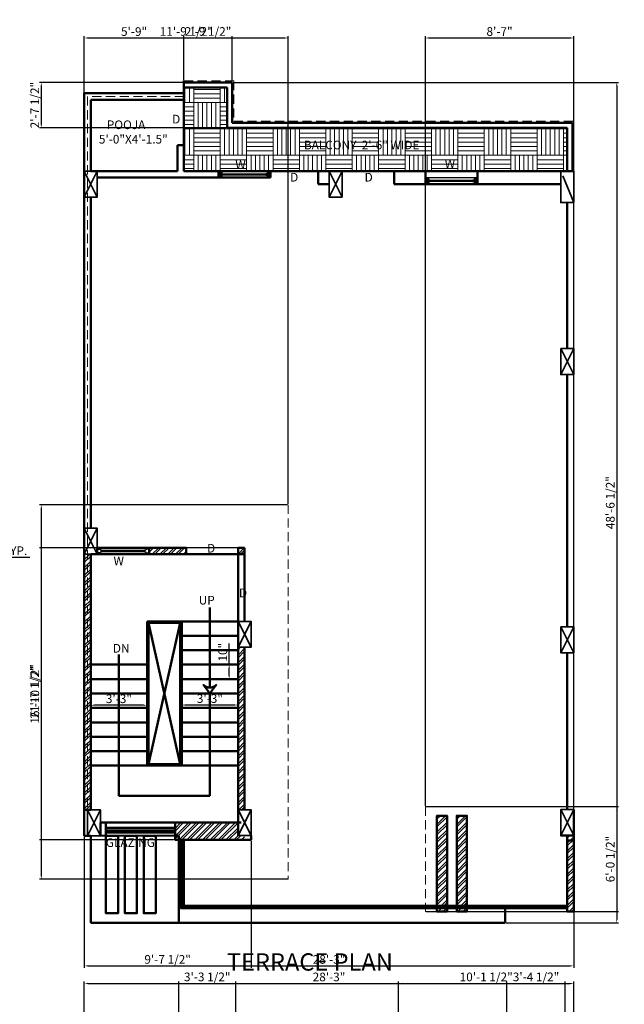
# Model space of a CAD drawing. Units: millimetres. Extents: x 67033 to 68301, y 155969 to 157209.
# Tile 17 of 17: x 67883 to 68301, y 156506 to 157188. Entities that reach past the tile are written whole.
import ezdxf

# ---------------------------------------------------------------- set-up
doc = ezdxf.new("R2010")
doc.units = ezdxf.units.MM
doc.linetypes.add('HIDDEN', pattern=[9.525, 6.35, -3.175])
for name, color, linetype, lineweight in [('A-ANNO-DIMS', 2, 'Continuous', 18), ('A-ANNO-TEXT', 7, 'Continuous', 18), ('A-AREA-IDEN', 3, 'Continuous', 18), ('A-COLS', 3, 'Continuous', 35), ('A-FLOR-OVHD', 1, 'HIDDEN', 18), ('A-FLOR-PATT', 252, 'Continuous', 13), ('A-GLAZ', 4, 'Continuous', 25), ('A-WALL', 7, 'Continuous', 50), ('A-WALL-PATT', 8, 'Continuous', 13)]:
    doc.layers.add(name, color=color, linetype=linetype, lineweight=lineweight)
doc.styles.get("Standard").update_dxf_attribs({"font": 'arial.ttf'})
doc.dimstyles.new('ISO-25', dxfattribs={"dimtxt": 6, "dimasz": 2.5, "dimexe": 1.25, "dimexo": 0.625, "dimtad": 1, "dimdec": 0, "dimlunit": 3, "dimtxsty": 'Standard', "dimcen": 2.5, "dimadec": 0, "dimazin": 0, "dimtfac": 1, "dimtdec": 0, "dimtmove": 0, "dimatfit": 3, "dimfxl": 1, "dimarcsym": 0})
pattern_1 = [(45, (858.7543, 0), (-2.69407684, 2.69407684), []), (45, (860.5504, 0), (-2.69407684, 2.69407684), [])]

# ---------------------------------------------------------------- blocks, each defined once
blk = doc.blocks.new('*D38')
at = {"layer": 'A-ANNO-DIMS', "color": 0, "lineweight": -2, "transparency": 16777216}
for p, q in [((67994.69, 156713.06), (67994.69, 156711.77)), ((68031.19, 156713.02), (67997.19, 156713.02)), ((68033.69, 156713.06), (68033.69, 156711.77))]:
    blk.add_line(p, q, dxfattribs=at)
at = {"layer": 'A-ANNO-DIMS', "color": 0, "transparency": 16777216}
for points in [[(67997.19, 156713.44), (67997.19, 156712.61), (67994.69, 156713.02)], [(68031.19, 156713.44), (68031.19, 156712.61), (68033.69, 156713.02)]]:
    blk.add_solid(points, dxfattribs=at)
at = {"layer": 'Defpoints', "color": 0, "transparency": 16777216}
for p in [(67994.69, 156713.68), (67994.69, 156713.02), (68033.69, 156713.68)]:
    blk.add_point(p, dxfattribs=at)
at = {"layer": 'A-ANNO-DIMS', "color": 0, "transparency": 16777216, "insert": (68014.19, 156716.71), "char_height": 6, "attachment_point": 5}
blk.add_mtext('3\'-3"', dxfattribs=at)
blk = doc.blocks.new('*D39')
at = {"layer": 'A-ANNO-DIMS', "color": 0, "lineweight": -2, "transparency": 16777216}
for p, q in [((67931.69, 156712.4), (67931.69, 156711.63)), ((67968.19, 156712.88), (67934.19, 156712.88)), ((67970.69, 156712.4), (67970.69, 156711.63))]:
    blk.add_line(p, q, dxfattribs=at)
at = {"layer": 'A-ANNO-DIMS', "color": 0, "transparency": 16777216}
for points in [[(67934.19, 156713.29), (67934.19, 156712.46), (67931.69, 156712.88)], [(67968.19, 156713.29), (67968.19, 156712.46), (67970.69, 156712.88)]]:
    blk.add_solid(points, dxfattribs=at)
at = {"layer": 'Defpoints', "color": 0, "transparency": 16777216}
for p in [(67931.69, 156713.02), (67931.69, 156712.88), (67970.69, 156713.02)]:
    blk.add_point(p, dxfattribs=at)
at = {"layer": 'A-ANNO-DIMS', "color": 0, "transparency": 16777216, "insert": (67951.19, 156716.57), "char_height": 6, "attachment_point": 5}
blk.add_mtext('3\'-3"', dxfattribs=at)
blk = doc.blocks.new('*D40')
at = {"layer": 'A-ANNO-DIMS', "color": 0, "lineweight": -2, "transparency": 16777216}
for p, q in [((68027.57, 156740.99), (68027.57, 156755.74)), ((68027.57, 156733.49), (68027.57, 156738.49)), ((68028.19, 156740.99), (68028.82, 156740.99)), ((68028.19, 156730.99), (68028.82, 156730.99))]:
    blk.add_line(p, q, dxfattribs=at)
at = {"layer": 'A-ANNO-DIMS', "color": 0, "transparency": 16777216}
for points in [[(68027.15, 156738.49), (68027.98, 156738.49), (68027.57, 156740.99)], [(68027.15, 156733.49), (68027.98, 156733.49), (68027.57, 156730.99)]]:
    blk.add_solid(points, dxfattribs=at)
at = {"layer": 'Defpoints', "color": 0, "transparency": 16777216}
for p in [(68027.57, 156740.99), (68027.57, 156740.99), (68027.57, 156730.99)]:
    blk.add_point(p, dxfattribs=at)
at = {"layer": 'A-ANNO-DIMS', "color": 0, "transparency": 16777216, "insert": (68023.88, 156749.62), "char_height": 6, "attachment_point": 5, "rotation": 90}
blk.add_mtext('10"', dxfattribs=at)
blk = doc.blocks.new('WIN-900')
for p, q in [((3.67, 3.22), (33.2, 3.22)), ((3.67, 2.74), (33.2, 2.74)), ((33.2, 2.27), (3.67, 2.27))]:
    blk.add_line(p, q)
blk.add_lwpolyline([(0.44, 4.99), (36.44, 4.99), (36.44, 0.49), (0.44, 0.49)], close=True)
for points in [[(0.44, 4.09), (2.73, 4.09), (2.73, 3.22), (3.67, 3.22), (3.67, 2.27), (2.73, 2.27), (2.73, 1.4), (0.44, 1.4)], [(36.44, 4.09), (34.14, 4.09), (34.14, 3.22), (33.2, 3.22), (33.2, 2.27), (34.14, 2.27), (34.14, 1.4), (36.44, 1.4)]]:
    blk.add_lwpolyline(points)
blk = doc.blocks.new('COLUMN-230x460')
for p, q in [((0.44, 17.99), (9.44, -0.01)), ((9.44, 17.99), (0.44, -0.01))]:
    blk.add_line(p, q)
blk.add_lwpolyline([(0.44, 17.99), (9.44, 17.99), (9.44, -0.01), (0.44, -0.01)], close=True)
blk = doc.blocks.new('COLUMN-TERR')
for p, q in [((9.32, 21.99), (9.32, 1.87)), ((1.64, 18.8), (9.32, 0.19))]:
    blk.add_line(p, q)
blk.add_lwpolyline([(0.32, 21.99), (9.32, 21.99), (9.32, 0.19), (0.32, 0.19)], close=True)
blk = doc.blocks.new('*D59')
at = {"layer": 'A-ANNO-DIMS', "color": 0, "lineweight": -2, "transparency": 16777216}
for p, q in [((67802.63, 156819.29), (67802.63, 156814.18)), ((67805.13, 156815.43), (67830.07, 156815.43)), ((67832.57, 156819.29), (67832.57, 156814.18)), ((67832.57, 156815.43), (67889.44, 156815.43))]:
    blk.add_line(p, q, dxfattribs=at)
at = {"layer": 'A-ANNO-DIMS', "color": 0, "transparency": 16777216}
for points in [[(67805.13, 156815.84), (67805.13, 156815.01), (67802.63, 156815.43)], [(67830.07, 156815.84), (67830.07, 156815.01), (67832.57, 156815.43)]]:
    blk.add_solid(points, dxfattribs=at)
at = {"layer": 'Defpoints', "color": 0, "transparency": 16777216}
for p in [(67802.63, 156819.92), (67832.57, 156819.92), (67832.57, 156815.43)]:
    blk.add_point(p, dxfattribs=at)
at = {"layer": 'A-ANNO-DIMS', "color": 0, "transparency": 16777216, "insert": (67862.26, 156819.15), "char_height": 6, "attachment_point": 5}
blk.add_mtext('WC 2\'-6" TYP.', dxfattribs=at)
blk = doc.blocks.new('*D117')
at = {"layer": 'A-ANNO-DIMS', "color": 0, "lineweight": -2, "transparency": 16777216}
for p, q in [((67927.19, 156621.85), (67927.19, 156531)), ((68266.19, 156569.34), (68266.19, 156531)), ((67929.69, 156532.25), (68263.69, 156532.25))]:
    blk.add_line(p, q, dxfattribs=at)
at = {"layer": 'A-ANNO-DIMS', "color": 0, "transparency": 16777216}
for points in [[(67929.69, 156532.66), (67929.69, 156531.83), (67927.19, 156532.25)], [(68263.69, 156532.66), (68263.69, 156531.83), (68266.19, 156532.25)]]:
    blk.add_solid(points, dxfattribs=at)
at = {"layer": 'Defpoints', "color": 0, "transparency": 16777216}
for p in [(67927.19, 156622.48), (68266.19, 156569.97), (68266.19, 156532.25)]:
    blk.add_point(p, dxfattribs=at)
at = {"layer": 'A-ANNO-DIMS', "color": 0, "transparency": 16777216, "insert": (68096.69, 156535.94), "char_height": 6, "attachment_point": 5}
blk.add_mtext('28\'-3"', dxfattribs=at)
blk = doc.blocks.new('*D118')
at = {"layer": 'A-ANNO-DIMS', "color": 0, "lineweight": -2, "transparency": 16777216}
for p, q in [((68030.32, 157144.49), (68297.19, 157144.49)), ((68295.94, 157141.99), (68295.94, 156564.5)), ((68219.36, 156562), (68297.19, 156562))]:
    blk.add_line(p, q, dxfattribs=at)
at = {"layer": 'A-ANNO-DIMS', "color": 0, "transparency": 16777216}
for points in [[(68295.52, 157141.99), (68296.36, 157141.99), (68295.94, 157144.49)], [(68295.52, 156564.5), (68296.36, 156564.5), (68295.94, 156562)]]:
    blk.add_solid(points, dxfattribs=at)
at = {"layer": 'Defpoints', "color": 0, "transparency": 16777216}
for p in [(68029.69, 157144.49), (68218.74, 156562), (68295.94, 156562)]:
    blk.add_point(p, dxfattribs=at)
at = {"layer": 'A-ANNO-DIMS', "color": 0, "transparency": 16777216, "insert": (68292.21, 156853.25), "char_height": 6, "attachment_point": 5, "rotation": 90}
blk.add_mtext('48\'-6 1/2"', dxfattribs=at)
blk = doc.blocks.new('*D119')
at = {"layer": 'A-ANNO-DIMS', "color": 0, "lineweight": -2, "transparency": 16777216}
for p, q in [((67927.19, 157137.62), (67927.19, 157176.49)), ((67929.69, 157175.24), (67993.69, 157175.24)), ((67996.19, 157146.12), (67996.19, 157176.49))]:
    blk.add_line(p, q, dxfattribs=at)
at = {"layer": 'A-ANNO-DIMS', "color": 0, "transparency": 16777216}
for points in [[(67929.69, 157175.66), (67929.69, 157174.83), (67927.19, 157175.24)], [(67993.69, 157175.66), (67993.69, 157174.83), (67996.19, 157175.24)]]:
    blk.add_solid(points, dxfattribs=at)
at = {"layer": 'Defpoints', "color": 0, "transparency": 16777216}
for p in [(67996.19, 157175.24), (67996.19, 157145.49), (67927.19, 157136.99)]:
    blk.add_point(p, dxfattribs=at)
at = {"layer": 'A-ANNO-DIMS', "color": 0, "transparency": 16777216, "insert": (67961.69, 157178.93), "char_height": 6, "attachment_point": 5}
blk.add_mtext('5\'-9"', dxfattribs=at)
blk = doc.blocks.new('*D120')
at = {"layer": 'A-ANNO-DIMS', "color": 0, "lineweight": -2, "transparency": 16777216}
for p, q in [((67996.19, 157146.12), (67996.19, 157176.49)), ((67998.69, 157175.24), (68027.19, 157175.24)), ((68029.69, 157145.12), (68029.69, 157176.49))]:
    blk.add_line(p, q, dxfattribs=at)
at = {"layer": 'A-ANNO-DIMS', "color": 0, "transparency": 16777216}
for points in [[(67998.69, 157175.66), (67998.69, 157174.83), (67996.19, 157175.24)], [(68027.19, 157175.66), (68027.19, 157174.83), (68029.69, 157175.24)]]:
    blk.add_solid(points, dxfattribs=at)
at = {"layer": 'Defpoints', "color": 0, "transparency": 16777216}
for p in [(68029.69, 157175.24), (67996.19, 157145.49), (68029.69, 157144.49)]:
    blk.add_point(p, dxfattribs=at)
at = {"layer": 'A-ANNO-DIMS', "color": 0, "transparency": 16777216, "insert": (68012.94, 157178.97), "char_height": 6, "attachment_point": 5}
blk.add_mtext('2\'-9 1/2"', dxfattribs=at)
blk = doc.blocks.new('*D121')
at = {"layer": 'A-ANNO-DIMS', "color": 0, "lineweight": -2, "transparency": 16777216}
for p, q in [((68029.07, 157144.49), (67896.19, 157144.49)), ((67897.44, 157141.99), (67897.44, 157115.49)), ((68025.57, 157112.99), (67896.19, 157112.99))]:
    blk.add_line(p, q, dxfattribs=at)
at = {"layer": 'A-ANNO-DIMS', "color": 0, "transparency": 16777216}
for points in [[(67897.02, 157141.99), (67897.86, 157141.99), (67897.44, 157144.49)], [(67897.02, 157115.49), (67897.86, 157115.49), (67897.44, 157112.99)]]:
    blk.add_solid(points, dxfattribs=at)
at = {"layer": 'Defpoints', "color": 0, "transparency": 16777216}
for p in [(68029.69, 157144.49), (67897.44, 157112.99), (68026.19, 157112.99)]:
    blk.add_point(p, dxfattribs=at)
at = {"layer": 'A-ANNO-DIMS', "color": 0, "transparency": 16777216, "insert": (67893.71, 157128.74), "char_height": 6, "attachment_point": 5, "rotation": 90}
blk.add_mtext('2\'-7 1/2"', dxfattribs=at)
blk = doc.blocks.new('*D122')
at = {"layer": 'A-ANNO-DIMS', "color": 0, "lineweight": -2, "transparency": 16777216}
for p, q in [((67927.19, 156621.85), (67927.19, 156531)), ((68042.69, 156618.85), (68042.69, 156531)), ((67929.69, 156532.25), (68040.19, 156532.25))]:
    blk.add_line(p, q, dxfattribs=at)
at = {"layer": 'A-ANNO-DIMS', "color": 0, "transparency": 16777216}
for points in [[(67929.69, 156532.66), (67929.69, 156531.83), (67927.19, 156532.25)], [(68040.19, 156532.66), (68040.19, 156531.83), (68042.69, 156532.25)]]:
    blk.add_solid(points, dxfattribs=at)
at = {"layer": 'Defpoints', "color": 0, "transparency": 16777216}
for p in [(67927.19, 156622.48), (68042.69, 156619.48), (68042.69, 156532.25)]:
    blk.add_point(p, dxfattribs=at)
at = {"layer": 'A-ANNO-DIMS', "color": 0, "transparency": 16777216, "insert": (67984.94, 156535.97), "char_height": 6, "attachment_point": 5}
blk.add_mtext('9\'-7 1/2"', dxfattribs=at)
blk = doc.blocks.new('*D123')
at = {"layer": 'A-ANNO-DIMS', "color": 0, "lineweight": -2, "transparency": 16777216}
for p, q in [((68037.57, 156821.99), (67896.19, 156821.99)), ((67897.44, 156819.49), (67897.44, 156621.98)), ((68042.07, 156619.48), (67896.19, 156619.48))]:
    blk.add_line(p, q, dxfattribs=at)
at = {"layer": 'A-ANNO-DIMS', "color": 0, "transparency": 16777216}
for points in [[(67897.02, 156819.49), (67897.86, 156819.49), (67897.44, 156821.99)], [(67897.02, 156621.98), (67897.86, 156621.98), (67897.44, 156619.48)]]:
    blk.add_solid(points, dxfattribs=at)
at = {"layer": 'Defpoints', "color": 0, "transparency": 16777216}
for p in [(68038.19, 156821.99), (67897.44, 156619.48), (68042.69, 156619.48)]:
    blk.add_point(p, dxfattribs=at)
at = {"layer": 'A-ANNO-DIMS', "color": 0, "transparency": 16777216, "insert": (67893.71, 156720.74), "char_height": 6, "attachment_point": 5, "rotation": 90}
blk.add_mtext('16\'-10 1/2"', dxfattribs=at)
blk = doc.blocks.new('*D124')
at = {"layer": 'A-ANNO-DIMS', "color": 0, "lineweight": -2, "transparency": 16777216}
for p, q in [((67927.19, 156852.46), (67927.19, 157176.49)), ((67929.69, 157175.24), (68065.98, 157175.24)), ((68068.48, 156852.46), (68068.48, 157176.49))]:
    blk.add_line(p, q, dxfattribs=at)
at = {"layer": 'A-ANNO-DIMS', "color": 0, "transparency": 16777216}
for points in [[(67929.69, 157175.66), (67929.69, 157174.83), (67927.19, 157175.24)], [(68065.98, 157175.66), (68065.98, 157174.83), (68068.48, 157175.24)]]:
    blk.add_solid(points, dxfattribs=at)
at = {"layer": 'Defpoints', "color": 0, "transparency": 16777216}
for p in [(68068.48, 157175.24), (67927.19, 156851.84), (68068.48, 156851.84)]:
    blk.add_point(p, dxfattribs=at)
at = {"layer": 'A-ANNO-DIMS', "color": 0, "transparency": 16777216, "insert": (67997.83, 157178.97), "char_height": 6, "attachment_point": 5}
blk.add_mtext('11\'-9 1/2"', dxfattribs=at)
blk = doc.blocks.new('*D125')
at = {"layer": 'A-ANNO-DIMS', "color": 0, "lineweight": -2, "transparency": 16777216}
for p, q in [((68067.85, 156851.84), (67896.19, 156851.84)), ((67897.44, 156849.34), (67897.44, 156594.74)), ((68067.85, 156592.24), (67896.19, 156592.24))]:
    blk.add_line(p, q, dxfattribs=at)
at = {"layer": 'A-ANNO-DIMS', "color": 0, "transparency": 16777216}
for points in [[(67897.02, 156849.34), (67897.86, 156849.34), (67897.44, 156851.84)], [(67897.02, 156594.74), (67897.86, 156594.74), (67897.44, 156592.24)]]:
    blk.add_solid(points, dxfattribs=at)
at = {"layer": 'Defpoints', "color": 0, "transparency": 16777216}
for p in [(68068.48, 156851.84), (67897.44, 156592.24), (68068.48, 156592.24)]:
    blk.add_point(p, dxfattribs=at)
at = {"layer": 'A-ANNO-DIMS', "color": 0, "transparency": 16777216, "insert": (67893.71, 156722.04), "char_height": 6, "attachment_point": 5, "rotation": 90}
blk.add_mtext('21\'-7 1/2"', dxfattribs=at)
blk = doc.blocks.new('*D126')
at = {"layer": 'A-ANNO-DIMS', "color": 0, "lineweight": -2, "transparency": 16777216}
for p, q in [((68163.39, 156643.26), (68163.39, 157176.49)), ((68165.89, 157175.24), (68263.69, 157175.24)), ((68266.19, 156641.12), (68266.19, 157176.49))]:
    blk.add_line(p, q, dxfattribs=at)
at = {"layer": 'A-ANNO-DIMS', "color": 0, "transparency": 16777216}
for points in [[(68165.89, 157175.66), (68165.89, 157174.83), (68163.39, 157175.24)], [(68263.69, 157175.66), (68263.69, 157174.83), (68266.19, 157175.24)]]:
    blk.add_solid(points, dxfattribs=at)
at = {"layer": 'Defpoints', "color": 0, "transparency": 16777216}
for p in [(68266.19, 157175.24), (68163.39, 156642.64), (68266.19, 156640.49)]:
    blk.add_point(p, dxfattribs=at)
at = {"layer": 'A-ANNO-DIMS', "color": 0, "transparency": 16777216, "insert": (68214.79, 157178.93), "char_height": 6, "attachment_point": 5}
blk.add_mtext('8\'-7"', dxfattribs=at)
blk = doc.blocks.new('*D127')
at = {"layer": 'A-ANNO-DIMS', "color": 0, "lineweight": -2, "transparency": 16777216}
for p, q in [((68164.01, 156642.64), (68297.19, 156642.64)), ((68295.94, 156640.14), (68295.94, 156572.47)), ((68164.01, 156569.97), (68297.19, 156569.97))]:
    blk.add_line(p, q, dxfattribs=at)
at = {"layer": 'A-ANNO-DIMS', "color": 0, "transparency": 16777216}
for points in [[(68295.52, 156640.14), (68296.36, 156640.14), (68295.94, 156642.64)], [(68295.52, 156572.47), (68296.36, 156572.47), (68295.94, 156569.97)]]:
    blk.add_solid(points, dxfattribs=at)
at = {"layer": 'Defpoints', "color": 0, "transparency": 16777216}
for p in [(68163.39, 156642.64), (68163.39, 156569.97), (68295.94, 156569.97)]:
    blk.add_point(p, dxfattribs=at)
at = {"layer": 'A-ANNO-DIMS', "color": 0, "transparency": 16777216, "insert": (68292.21, 156606.3), "char_height": 6, "attachment_point": 5, "rotation": 90}
blk.add_mtext('6\'-0 1/2"', dxfattribs=at)
blk = doc.blocks.new('*D128')
at = {"layer": 'A-ANNO-DIMS', "color": 0, "lineweight": -2, "transparency": 16777216}
for p, q in [((67927.19, 156486.82), (67927.19, 156521.36)), ((67929.69, 156520.11), (68263.69, 156520.11)), ((68266.19, 156418.82), (68266.19, 156521.36))]:
    blk.add_line(p, q, dxfattribs=at)
at = {"layer": 'A-ANNO-DIMS', "color": 0, "transparency": 16777216}
for points in [[(67929.69, 156520.52), (67929.69, 156519.69), (67927.19, 156520.11)], [(68263.69, 156520.52), (68263.69, 156519.69), (68266.19, 156520.11)]]:
    blk.add_solid(points, dxfattribs=at)
at = {"layer": 'Defpoints', "color": 0, "transparency": 16777216}
for p in [(68266.19, 156520.11), (67927.19, 156486.2), (68266.19, 156418.2)]:
    blk.add_point(p, dxfattribs=at)
at = {"layer": 'A-ANNO-DIMS', "color": 0, "transparency": 16777216, "insert": (68096.69, 156523.8), "char_height": 6, "attachment_point": 5}
blk.add_mtext('28\'-3"', dxfattribs=at)
blk = doc.blocks.new('*D144')
at = {"layer": 'A-ANNO-DIMS', "color": 0, "lineweight": -2, "transparency": 16777216}
for p, q in [((67992.65, 156495.23), (67992.65, 156521.36)), ((67995.15, 156520.11), (68029.57, 156520.11)), ((68032.07, 156495.23), (68032.07, 156521.36))]:
    blk.add_line(p, q, dxfattribs=at)
at = {"layer": 'A-ANNO-DIMS', "color": 0, "transparency": 16777216}
for points in [[(67995.15, 156520.52), (67995.15, 156519.69), (67992.65, 156520.11)], [(68029.57, 156520.52), (68029.57, 156519.69), (68032.07, 156520.11)]]:
    blk.add_solid(points, dxfattribs=at)
at = {"layer": 'Defpoints', "color": 0, "transparency": 16777216}
for p in [(68032.07, 156520.11), (67992.65, 156494.61), (68032.07, 156494.61)]:
    blk.add_point(p, dxfattribs=at)
at = {"layer": 'A-ANNO-DIMS', "color": 0, "transparency": 16777216, "insert": (68012.36, 156523.84), "char_height": 6, "attachment_point": 5}
blk.add_mtext('3\'-3 1/2"', dxfattribs=at)
blk = doc.blocks.new('*D145')
at = {"layer": 'A-ANNO-DIMS', "color": 0, "lineweight": -2, "transparency": 16777216}
for p, q in [((68144.87, 156418.82), (68144.87, 156521.36)), ((68147.37, 156520.11), (68263.69, 156520.11)), ((68266.19, 156418.82), (68266.19, 156521.36))]:
    blk.add_line(p, q, dxfattribs=at)
at = {"layer": 'A-ANNO-DIMS', "color": 0, "transparency": 16777216}
for points in [[(68147.37, 156520.52), (68147.37, 156519.69), (68144.87, 156520.11)], [(68263.69, 156520.52), (68263.69, 156519.69), (68266.19, 156520.11)]]:
    blk.add_solid(points, dxfattribs=at)
at = {"layer": 'Defpoints', "color": 0, "transparency": 16777216}
for p in [(68266.19, 156520.11), (68144.87, 156418.2), (68266.19, 156418.2)]:
    blk.add_point(p, dxfattribs=at)
at = {"layer": 'A-ANNO-DIMS', "color": 0, "transparency": 16777216, "insert": (68205.53, 156523.83), "char_height": 6, "attachment_point": 5}
blk.add_mtext('10\'-1 1/2"', dxfattribs=at)
blk = doc.blocks.new('*D146')
at = {"layer": 'A-ANNO-DIMS', "color": 0, "lineweight": -2, "transparency": 16777216}
for p, q in [((68219.91, 156350.82), (68219.91, 156521.36)), ((68222.41, 156520.11), (68257.69, 156520.11)), ((68260.19, 156396.82), (68260.19, 156521.36))]:
    blk.add_line(p, q, dxfattribs=at)
at = {"layer": 'A-ANNO-DIMS', "color": 0, "transparency": 16777216}
for points in [[(68222.41, 156520.52), (68222.41, 156519.69), (68219.91, 156520.11)], [(68257.69, 156520.52), (68257.69, 156519.69), (68260.19, 156520.11)]]:
    blk.add_solid(points, dxfattribs=at)
at = {"layer": 'Defpoints', "color": 0, "transparency": 16777216}
for p in [(68260.19, 156520.11), (68260.19, 156396.2), (68219.91, 156350.2)]:
    blk.add_point(p, dxfattribs=at)
at = {"layer": 'A-ANNO-DIMS', "color": 0, "transparency": 16777216, "insert": (68240.05, 156523.84), "char_height": 6, "attachment_point": 5}
blk.add_mtext('3\'-4 1/2"', dxfattribs=at)

msp = doc.modelspace()

# ---------------------------------------------------------------- hatches: boundary and pattern name
at = {"layer": 'A-FLOR-PATT'}
h = msp.add_hatch(dxfattribs=at)
h.set_pattern_fill('AR-PARQ1', color=256, scale=0.06)
h.set_pattern_definition([(90, (428.876, 0), (-18.288, 18.288), [18.288, -18.288]), (90, (431.924, 0), (-18.288, 18.288), [18.288, -18.288]), (90, (434.972, 0), (-18.288, 18.288), [18.288, -18.288]), (90, (438.02, 0), (-18.288, 18.288), [18.288, -18.288]), (90, (441.068, 0), (-18.288, 18.288), [18.288, -18.288]), (90, (444.116, 0), (-18.288, 18.288), [18.288, -18.288]), (90, (447.164, 0), (-18.288, 18.288), [18.288, -18.288]), (0, (428.876, 18.288), (18.288, -18.288), [18.288, -18.288]), (0, (428.876, 21.336), (18.288, -18.288), [18.288, -18.288]), (0, (428.876, 24.384), (18.288, -18.288), [18.288, -18.288]), (0, (428.876, 27.432), (18.288, -18.288), [18.288, -18.288]), (0, (428.876, 30.48), (18.288, -18.288), [18.288, -18.288]), (0, (428.876, 33.528), (18.288, -18.288), [18.288, -18.288]), (0, (428.876, 36.576), (18.288, -18.288), [18.288, -18.288])])
h.paths.add_polyline_path([(68261.69, 157112.99), (68026.19, 157112.99), (68026.19, 157140.99), (67996.19, 157140.99), (67996.19, 157082.99), (68056.19, 157082.99), (68089.19, 157082.99), (68261.69, 157082.99)])
h.paths.add_polyline_path([(68024.82, 157081.09), (68042.71, 157081.09), (68042.71, 157093.46), (68024.82, 157093.46)], flags=9)
h.paths.add_polyline_path([(68169.82, 157081.83), (68187.72, 157081.83), (68187.72, 157094.2), (68169.82, 157094.2)], flags=9)
at = {"layer": 'A-GLAZ'}
h = msp.add_hatch(color=256, dxfattribs=at)
h.dxf.hatch_style = 1
h.paths.add_polyline_path([(68023.43, 157081.22), (68022.49, 157081.22), (68022.49, 157082.09), (68020.19, 157082.09), (68020.19, 157079.4), (68022.49, 157079.4), (68022.49, 157080.27), (68023.43, 157080.27)])
h = msp.add_hatch(color=256, dxfattribs=at)
h.dxf.hatch_style = 1
h.paths.add_polyline_path([(68056.19, 157082.09), (68053.89, 157082.09), (68053.89, 157081.22), (68052.95, 157081.22), (68052.95, 157080.27), (68053.89, 157080.27), (68053.89, 157079.4), (68056.19, 157079.4)])
h = msp.add_hatch(color=256, dxfattribs=at)
h.dxf.hatch_style = 1
h.paths.add_polyline_path([(68166.68, 157076.72), (68165.74, 157076.72), (68165.74, 157077.59), (68163.44, 157077.59), (68163.44, 157074.9), (68165.74, 157074.9), (68165.74, 157075.77), (68166.68, 157075.77)])
h = msp.add_hatch(color=256, dxfattribs=at)
h.dxf.hatch_style = 1
h.paths.add_polyline_path([(68199.44, 157077.59), (68197.14, 157077.59), (68197.14, 157076.72), (68196.2, 157076.72), (68196.2, 157075.77), (68197.14, 157075.77), (68197.14, 157074.9), (68199.44, 157074.9)])
at = {"layer": 'A-WALL-PATT'}
h = msp.add_hatch(dxfattribs=at)
h.set_pattern_fill('ANSI32', color=256, scale=0.4)
h.set_pattern_definition(pattern_1)
h.paths.add_polyline_path([(67997.69, 156821.99), (67972.19, 156821.99), (67972.19, 156817.49), (67997.69, 156817.49)])
h = msp.add_hatch(dxfattribs=at)
h.set_pattern_fill('ANSI32', color=256, scale=0.4)
h.set_pattern_definition(pattern_1)
h.paths.add_polyline_path([(68038.19, 156821.99), (68033.69, 156821.99), (68033.69, 156817.49), (68038.19, 156817.49)])
h = msp.add_hatch(dxfattribs=at)
h.set_pattern_fill('ANSI32', color=256, scale=0.4)
h.set_pattern_definition(pattern_1)
h.paths.add_polyline_path([(67931.69, 156817.49), (67927.19, 156817.49), (67927.19, 156640.48), (67931.69, 156640.48)])
h = msp.add_hatch(dxfattribs=at)
h.set_pattern_fill('ANSI32', color=256, scale=0.4)
h.set_pattern_definition(pattern_1)
h.paths.add_polyline_path([(68038.19, 156752.99), (68033.69, 156752.99), (68033.69, 156640.48), (68038.19, 156640.48)])
h = msp.add_hatch(dxfattribs=at)
h.set_pattern_fill('ANSI32', color=256, scale=0.4)
h.set_pattern_definition([(45, (997.897, -72.8208), (-2.69407684, 2.69407684), []), (45, (999.693, -72.8208), (-2.69407684, 2.69407684), [])])
h.paths.add_polyline_path([(68178.44, 156636.25), (68171.46, 156636.25), (68171.46, 156569.97), (68178.44, 156569.97)])
h = msp.add_hatch(dxfattribs=at)
h.set_pattern_fill('ANSI32', color=256, scale=0.4)
h.set_pattern_definition([(45, (1011.601, -72.8208), (-2.69407684, 2.69407684), []), (45, (1013.397, -72.8208), (-2.69407684, 2.69407684), [])])
h.paths.add_polyline_path([(68192.14, 156636.25), (68185.16, 156636.25), (68185.16, 156569.97), (68192.14, 156569.97)])
h = msp.add_hatch(dxfattribs=at)
h.set_pattern_fill('ANSI32', color=256, scale=0.4)
h.set_pattern_definition([(45, (428.876, 0), (-2.69407684, 2.69407684), []), (45, (430.672, 0), (-2.69407684, 2.69407684), [])])
h.paths.add_polyline_path([(68033.69, 156631.49), (67990.19, 156631.49), (67990.19, 156622.48), (67990.19, 156619.48), (68038.19, 156619.48), (68038.19, 156622.48), (68033.68, 156622.48), (68033.69, 156622.49)])
h = msp.add_hatch(dxfattribs=at)
h.set_pattern_fill('ANSI32', color=256, scale=0.4)
h.set_pattern_definition([(45, (1086.7543, -81.8886), (-2.69407684, 2.69407684), []), (45, (1088.5504, -81.8886), (-2.69407684, 2.69407684), [])])
h.paths.add_polyline_path([(68266.19, 156622.49), (68261.69, 156622.49), (68261.69, 156569.97), (68266.19, 156569.97)])

# ---------------------------------------------------------------- linework, layer by layer
at = {"layer": 'A-FLOR-OVHD'}
for p, q in [((67996.19, 157145.49), (68030.69, 157145.49)), ((68030.69, 157145.49), (68030.69, 157117.49)), ((67996.19, 157134.69), (67929.37, 157134.7)), ((67929.37, 157134.7), (67929.37, 156622.48)), ((68030.69, 157117.49), (68266.19, 157117.49)), ((68266.19, 157082.99), (68266.19, 157117.49)), ((68266.19, 156640.49), (68266.19, 157061.19)), ((67927.19, 156851.84), (68068.48, 156851.84)), ((68068.48, 156851.84), (68068.48, 156592.24)), ((68261.69, 156642.64), (68163.39, 156642.64)), ((68163.39, 156642.64), (68163.39, 156569.97)), ((67931.69, 156592.24), (68068.48, 156592.24)), ((68163.39, 156569.97), (68261.69, 156569.97))]:
    msp.add_line(p, q, dxfattribs=at)
at = {"layer": 'A-WALL'}
for p, q in [((67996.19, 157145.49), (67996.19, 157082.99)), ((67996.19, 157144.49), (68029.69, 157144.49)), ((67996.19, 157140.99), (68026.19, 157140.99)), ((68026.19, 157140.99), (68026.19, 157112.99)), ((68029.69, 157144.49), (68029.69, 157116.49)), ((67927.19, 157136.99), (67927.19, 156622.48)), ((67996.19, 157136.99), (67927.19, 157136.99)), ((67996.19, 157134.69), (67996.19, 157134.69)), ((67931.69, 157132.49), (67931.69, 157082.99)), ((67931.69, 157132.49), (67996.19, 157132.49)), ((68029.69, 157116.49), (68265.19, 157116.49)), ((68265.19, 157116.49), (68265.19, 157082.99)), ((68026.19, 157112.99), (68261.69, 157112.99)), ((68261.69, 157112.99), (68261.69, 157082.99)), ((67991.69, 157100.99), (67991.69, 157082.99)), ((67991.69, 157100.99), (67996.19, 157100.99)), ((67931.69, 157082.99), (67991.69, 157082.99)), ((67996.19, 157082.99), (68056.19, 157082.99)), ((68020.19, 157082.99), (68020.19, 157078.49)), ((68056.19, 157082.99), (68056.19, 157078.49)), ((68056.19, 157082.99), (68089.19, 157082.99)), ((68089.19, 157082.99), (68089.19, 157073.99)), ((68089.19, 157082.99), (68266.19, 157082.99)), ((68141.69, 157082.99), (68141.69, 157073.99)), ((68163.44, 157073.99), (68163.44, 157082.99)), ((68199.44, 157073.99), (68199.44, 157082.99)), ((67936.19, 157078.49), (68056.19, 157078.49)), ((68089.19, 157073.99), (68096.69, 157073.99)), ((68141.69, 157073.99), (68257.19, 157073.99)), ((68163.44, 157078.49), (68163.44, 157073.99)), ((68199.44, 157078.49), (68199.44, 157073.99)), ((67931.69, 157064.99), (67931.69, 156835.49)), ((68261.69, 157061.19), (68261.69, 156959.99)), ((68261.69, 156941.99), (68261.69, 156767.19)), ((67936.19, 156821.99), (67997.69, 156821.99)), ((67936.19, 156821.99), (67936.19, 156817.49)), ((67972.19, 156821.99), (67972.19, 156817.49)), ((67997.69, 156821.99), (67997.69, 156817.49)), ((68033.69, 156821.99), (68033.69, 156622.49)), ((68033.69, 156821.99), (68038.19, 156821.99)), ((68038.19, 156770.99), (68038.19, 156821.99)), ((67931.69, 156817.49), (67931.69, 156640.48)), ((67931.69, 156817.49), (67997.69, 156817.49)), ((68033.69, 156817.49), (67997.69, 156817.49)), ((68033.69, 156817.49), (68038.19, 156817.49)), ((68014.19, 156725.08), (68014.19, 156780.67)), ((67970.69, 156770.99), (67970.69, 156670.99)), ((67970.69, 156770.99), (68033.69, 156770.99)), ((67971.69, 156769.99), (67971.69, 156671.99)), ((67971.69, 156769.99), (67993.69, 156769.99)), ((67993.69, 156769.99), (67971.69, 156671.99)), ((67971.69, 156769.99), (67993.69, 156671.99)), ((67993.69, 156769.99), (67993.69, 156671.99)), ((67994.69, 156770.99), (67994.69, 156670.99)), ((67994.69, 156760.99), (68033.69, 156760.99)), ((68038.19, 156752.99), (68038.19, 156640.48)), ((67951.19, 156747.98), (67951.19, 156650.15)), ((67994.69, 156750.99), (68033.69, 156750.99)), ((68261.69, 156749.19), (68261.69, 156689.99)), ((67931.69, 156740.99), (67970.69, 156740.99)), ((67994.69, 156740.99), (68033.69, 156740.99)), ((67931.69, 156730.99), (67970.69, 156730.99)), ((67994.69, 156730.99), (68033.69, 156730.99)), ((67931.69, 156720.99), (67970.69, 156720.99)), ((67994.69, 156720.99), (68033.69, 156720.99)), ((68014.19, 156720.99), (68014.19, 156650.15)), ((67931.69, 156710.99), (67970.69, 156710.99)), ((67994.69, 156710.99), (68033.69, 156710.99)), ((67931.69, 156700.99), (67970.69, 156700.99)), ((67994.69, 156700.99), (68033.69, 156700.99)), ((67931.69, 156690.99), (67970.69, 156690.99)), ((67994.69, 156690.99), (68033.69, 156690.99)), ((68261.69, 156689.99), (68261.69, 156685.49)), ((68261.69, 156685.49), (68261.69, 156640.49)), ((67931.69, 156680.99), (67970.69, 156680.99)), ((67994.69, 156680.99), (68033.69, 156680.99)), ((67931.69, 156670.99), (67994.69, 156670.99)), ((67971.69, 156671.99), (67993.69, 156671.99)), ((67994.69, 156670.99), (68033.69, 156670.99)), ((67951.19, 156650.15), (68014.19, 156650.15)), ((67931.69, 156640.48), (67927.19, 156640.48)), ((68266.19, 156640.49), (68266.19, 156569.97)), ((68035.87, 156631.49), (67938.37, 156631.49)), ((67938.37, 156631.48), (67938.37, 156622.48)), ((67942.19, 156631.48), (67942.19, 156622.48)), ((67990.19, 156631.48), (67990.19, 156622.48)), ((67931.69, 156622.48), (67927.19, 156622.48)), ((67931.69, 156622.48), (67931.69, 156562)), ((67938.37, 156622.48), (67992.37, 156622.49)), ((67942.19, 156627.98), (67990.19, 156627.98)), ((67942.19, 156625.98), (67990.19, 156625.98)), ((67942.19, 156624.61), (67990.19, 156624.61)), ((67990.19, 156622.48), (67990.19, 156619.48)), ((67992.65, 156622.48), (67992.65, 156562)), ((68042.69, 156619.48), (68042.69, 156622.49)), ((68257.19, 156622.49), (68266.19, 156622.49)), ((68261.69, 156622.49), (68261.69, 156569.97)), ((67990.19, 156619.48), (68042.69, 156619.48)), ((67993.83, 156619.48), (67993.83, 156572.15)), ((67994.83, 156573.05), (67994.83, 156619.48)), ((67996.05, 156573.95), (67996.05, 156619.48)), ((68261.69, 156619.06), (68266.19, 156619.06)), ((68261.69, 156572.15), (67993.83, 156572.15)), ((68261.69, 156573.05), (67994.83, 156573.05)), ((68261.69, 156573.95), (67996.05, 156573.95)), ((68218.74, 156572.15), (68218.74, 156562)), ((68261.69, 156569.97), (68266.19, 156569.97)), ((68218.74, 156562), (67931.69, 156562))]:
    msp.add_line(p, q, dxfattribs=at)
msp.add_lwpolyline([(68014.19, 156720.99), (68009.73, 156726.93, 0.414166), (68018.65, 156726.93)], format="xyb", close=True, dxfattribs=at)
for points in [[(68171.46, 156569.97), (68178.44, 156569.97), (68178.44, 156636.25), (68171.46, 156636.25)], [(68185.16, 156569.97), (68192.14, 156569.97), (68192.14, 156636.25), (68185.16, 156636.25)], [(67942.19, 156622.48), (67950.57, 156622.48), (67950.57, 156568.7), (67942.19, 156568.7)], [(67955.32, 156622.48), (67963.7, 156622.48), (67963.7, 156568.7), (67955.32, 156568.7)], [(67968.38, 156622.48), (67976.76, 156622.48), (67976.76, 156568.7), (67968.38, 156568.7)]]:
    msp.add_lwpolyline(points, close=True, dxfattribs=at)

# ---------------------------------------------------------------- block references
at = {"layer": 'A-COLS'}
for name, p in [('COLUMN-230x460', (67926.75, 157065)), ('COLUMN-230x460', (68096.25, 157065)), ('COLUMN-TERR', (68256.88, 157061)), ('COLUMN-230x460', (68256.75, 156942)), ('COLUMN-230x460', (67926.75, 156817.5)), ('COLUMN-230x460', (68033.25, 156753)), ('COLUMN-230x460', (68256.75, 156749.2))]:
    msp.add_blockref(name, p, dxfattribs=at)
for p, rotation in [((67928.94, 156622.49), 359.9276884764716), ((68266.63, 156640.49), 180)]:
    msp.add_blockref('COLUMN-230x460', p, dxfattribs=dict(at, rotation=rotation))
at = {"layer": 'A-COLS', "extrusion": (0, 0, -1), "zscale": -1, "rotation": 180.0076170380899}
msp.add_blockref('COLUMN-230x460', (-68033.26, 156640.48), dxfattribs=at)
at = {"layer": 'A-GLAZ'}
for p in [(68019.75, 157078), (68163, 157073.5), (67935.75, 156817)]:
    msp.add_blockref('WIN-900', p, dxfattribs=at)

# ---------------------------------------------------------------- texts
at = {"layer": 'A-ANNO-TEXT', "attachment_point": 1}
for s, width, insert, char_height in [('   D', 19.5287, (67982.56, 157121.99), 6), ('   W', 19.5287, (68026.32, 157090.37), 6), ('   W', 19.5287, (68171.32, 157091.11), 6), ('   D', 19.5287, (68064.27, 157081.74), 6), ('   D', 19.5287, (68115.85, 157081.74), 6), ('   D', 19.5287, (68006.73, 156824.67), 6), ('   W', 19.5287, (67941.98, 156815.8), 6), ('   D', 19.5287, (68028.81, 156793.68), 6), (' UP', 19.5287, (68004.65, 156788.65), 6), (' DN', 19.5287, (67945.19, 156755.33), 6), ('TERRACE PLAN', 203.6887, (68025.94, 156540.96), 12)]:
    msp.add_mtext_dynamic_manual_height_columns(s, width=width, gutter_width=12.5, heights=[0], dxfattribs=dict(at, insert=insert, char_height=char_height))
at = {"layer": 'A-AREA-IDEN', "char_height": 6, "attachment_point": 1}
for s, width, insert in [('       POOJA \\P    5\'-0"X4\'-1.5"', 59.4046, (67929.99, 157118.1)), (' BALCONY  2\'-6" WIDE', 93.5859, (68077.46, 157104.08)), ('    GLAZING', 59.4046, (67934.83, 156620.64))]:
    msp.add_mtext_dynamic_manual_height_columns(s, width=width, gutter_width=12.5, heights=[0], dxfattribs=dict(at, insert=insert))

# ---------------------------------------------------------------- dimensions: what is measured, and where the dimension line sits
at = {"layer": 'A-ANNO-DIMS'}
for base, p1, p2, override, picture, middle in [((68068.48, 157175.24), (67927.19, 156851.84), (68068.48, 156851.84), {"dimdec": 1, "dimlfac": 1, "dimrnd": 0, "dimzin": 1, "dimdsep": 46, "dimlunit": 4, "dimfrac": 2}, '*D124', (67997.83, 157178.97)), ((67996.19, 157175.24), (67927.19, 157136.99), (67996.19, 157145.49), {"dimdec": 1, "dimlfac": 1, "dimrnd": 0, "dimzin": 1, "dimdsep": 46, "dimlunit": 4, "dimfrac": 2}, '*D119', (67961.69, 157178.93)), ((68029.69, 157175.24), (67996.19, 157145.49), (68029.69, 157144.49), {"dimdec": 1, "dimlfac": 1, "dimrnd": 0, "dimzin": 1, "dimdsep": 46, "dimlunit": 4, "dimfrac": 2}, '*D120', (68012.94, 157178.97)), ((68266.19, 157175.24), (68163.39, 156642.64), (68266.19, 156640.49), {"dimdec": 1, "dimlfac": 1, "dimrnd": 0, "dimzin": 1, "dimdsep": 46, "dimlunit": 4, "dimfrac": 2}, '*D126', (68214.79, 157178.93)), ((67931.69, 156712.88), (67970.69, 156713.02), (67931.69, 156713.02), {"dimclrd": 0, "dimclre": 0, "dimclrt": 0}, '*D39', (67951.19, 156716.57)), ((67994.69, 156713.02), (68033.69, 156713.68), (67994.69, 156713.68), {"dimclrd": 0, "dimclre": 0, "dimclrt": 0}, '*D38', (68014.19, 156716.71)), ((68266.19, 156532.25), (67927.19, 156622.48), (68266.19, 156569.97), {"dimdec": 1, "dimlfac": 1, "dimrnd": 0, "dimzin": 1, "dimdsep": 46, "dimlunit": 4, "dimfrac": 2}, '*D117', (68096.69, 156535.94)), ((68042.69, 156532.25), (67927.19, 156622.48), (68042.69, 156619.48), {"dimdec": 1, "dimlfac": 1, "dimrnd": 0, "dimzin": 1, "dimdsep": 46, "dimlunit": 4, "dimfrac": 2}, '*D122', (67984.94, 156535.97)), ((68266.19, 156520.11), (67927.19, 156486.2), (68266.19, 156418.2), {"dimdec": 1, "dimlfac": 1, "dimrnd": 0, "dimzin": 1, "dimdsep": 46, "dimlunit": 4, "dimfrac": 2}, '*D128', (68096.69, 156523.8)), ((68032.07, 156520.11), (67992.65, 156494.61), (68032.07, 156494.61), {"dimdec": 1, "dimlfac": 1, "dimrnd": 0, "dimzin": 1, "dimdsep": 46, "dimlunit": 4, "dimfrac": 2}, '*D144', (68012.36, 156523.84)), ((68266.19, 156520.11), (68144.87, 156418.2), (68266.19, 156418.2), {"dimdec": 1, "dimlfac": 1, "dimrnd": 0, "dimzin": 1, "dimdsep": 46, "dimlunit": 4, "dimfrac": 2}, '*D145', (68205.53, 156523.83)), ((68260.19, 156520.11), (68219.91, 156350.2), (68260.19, 156396.2), {"dimdec": 1, "dimlfac": 1, "dimrnd": 0, "dimzin": 1, "dimdsep": 46, "dimlunit": 4, "dimfrac": 2}, '*D146', (68240.05, 156523.84))]:
    dim = msp.add_linear_dim(base=base, p1=p1, p2=p2, dimstyle='ISO-25', override=override, dxfattribs=at)
    dim.commit()
    dim.dimension.update_dxf_attribs({"geometry": picture, "text_midpoint": middle})
for base, p1, p2, override, picture, middle in [((67897.44, 157112.99), (68029.69, 157144.49), (68026.19, 157112.99), {"dimdec": 1, "dimlfac": 1, "dimrnd": 0, "dimzin": 1, "dimdsep": 46, "dimlunit": 4, "dimfrac": 2}, '*D121', (67893.71, 157128.74)), ((68295.94, 156562), (68029.69, 157144.49), (68218.74, 156562), {"dimdec": 1, "dimlfac": 1, "dimrnd": 0, "dimzin": 1, "dimdsep": 46, "dimlunit": 4, "dimfrac": 2}, '*D118', (68292.21, 156853.25)), ((67897.44, 156592.24), (68068.48, 156851.84), (68068.48, 156592.24), {"dimdec": 1, "dimlfac": 1, "dimrnd": 0, "dimzin": 1, "dimdsep": 46, "dimlunit": 4, "dimfrac": 2}, '*D125', (67893.71, 156722.04)), ((67897.44, 156619.48), (68038.19, 156821.99), (68042.69, 156619.48), {"dimdec": 1, "dimlfac": 1, "dimrnd": 0, "dimzin": 1, "dimdsep": 46, "dimlunit": 4, "dimfrac": 2}, '*D123', (67893.71, 156720.74)), ((68027.57, 156740.99), (68027.57, 156730.99), (68027.57, 156740.99), {"dimclrd": 0, "dimclre": 0, "dimclrt": 0}, '*D40', (68023.88, 156749.62)), ((68295.94, 156569.97), (68163.39, 156642.64), (68163.39, 156569.97), {"dimdec": 1, "dimlfac": 1, "dimrnd": 0, "dimzin": 1, "dimdsep": 46, "dimlunit": 4, "dimfrac": 2}, '*D127', (68292.21, 156606.3))]:
    dim = msp.add_linear_dim(base=base, p1=p1, p2=p2, angle=90, dimstyle='ISO-25', override=override, dxfattribs=at)
    dim.commit()
    dim.dimension.update_dxf_attribs({"geometry": picture, "text_midpoint": middle})
dim = msp.add_linear_dim(base=(67832.57, 156815.43), p1=(67802.63, 156819.92), p2=(67832.57, 156819.92), text='WC <> TYP.', dimstyle='ISO-25', override={"dimdec": 1, "dimrnd": 0, "dimzin": 1, "dimlunit": 4, "dimfrac": 2}, dxfattribs=at)
dim.commit()
dim.dimension.update_dxf_attribs({"geometry": '*D59', "text_midpoint": (67862.26, 156819.15)})

doc.saveas('drawing.dxf')
